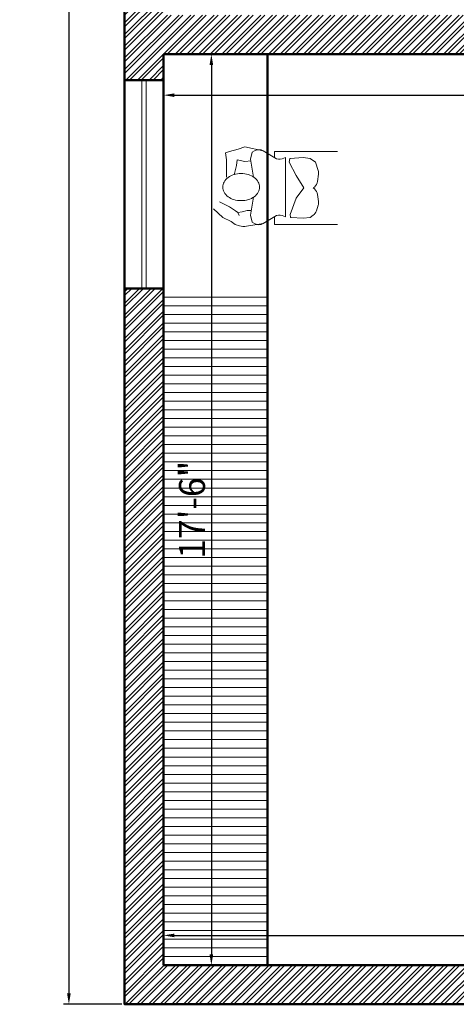
# Model space of a CAD drawing. Units: inches. Extents: x 3590 to 5167, y 65 to 1917.
# Tile 1 of 100: x 3621 to 3722, y 109 to 336. Entities that reach past the tile are written whole.
import ezdxf

# ---------------------------------------------------------------- set-up
doc = ezdxf.new("R2010")
doc.units = ezdxf.units.IN
for name, color, linetype, lineweight in [('A-ANNO-DIMS', 2, 'Continuous', 18), ('A-FURN', 21, 'Continuous', 18), ('A-GLAZ', 4, 'Continuous', 18), ('A-WALL', 7, 'Continuous', 50), ('A-WALL-PATT', 251, 'Continuous', 13)]:
    doc.layers.add(name, color=color, linetype=linetype, lineweight=lineweight)
doc.styles.get("Standard").update_dxf_attribs({"font": 'arial.ttf'})
doc.dimstyles.new('ISO-25', dxfattribs={"dimtxt": 9, "dimasz": 2.5, "dimexe": 1.25, "dimexo": 0.625, "dimtad": 1, "dimdec": 1, "dimlunit": 3, "dimtxsty": 'Standard', "dimcen": 2.5, "dimadec": 0, "dimazin": 0, "dimtfac": 1, "dimtdec": 1, "dimtmove": 0, "dimatfit": 3, "dimfxl": 1, "dimarcsym": 0})

# ---------------------------------------------------------------- blocks, each defined once
blk = doc.blocks.new('*D248')
at = {"layer": 'A-ANNO-DIMS', "color": 0, "lineweight": -2, "transparency": 16777216}
for p, q in [((3644.89, 589.06), (3631.39, 589.06)), ((3632.64, 586.56), (3632.64, 111.56)), ((3644.89, 109.06), (3631.39, 109.06))]:
    blk.add_line(p, q, dxfattribs=at)
at = {"layer": 'A-ANNO-DIMS', "color": 0, "transparency": 16777216}
for points in [[(3632.22, 586.56), (3633.06, 586.56), (3632.64, 589.06)], [(3632.22, 111.56), (3633.06, 111.56), (3632.64, 109.06)]]:
    blk.add_solid(points, dxfattribs=at)
at = {"layer": 'Defpoints', "color": 0, "transparency": 16777216}
for p in [(3645.51, 589.06), (3632.64, 109.06), (3645.51, 109.06)]:
    blk.add_point(p, dxfattribs=at)
at = {"layer": 'A-ANNO-DIMS', "color": 0, "transparency": 16777216, "insert": (3627.42, 349.06), "char_height": 9, "attachment_point": 5, "rotation": 90}
blk.add_mtext("40'", dxfattribs=at)
blk = doc.blocks.new('*D240')
at = {"layer": 'A-ANNO-DIMS', "color": 0, "lineweight": -2, "transparency": 16777216}
for p, q in [((3654.51, 327.43), (3654.51, 317.35)), ((3864.51, 327.43), (3864.51, 317.35)), ((3657.01, 318.6), (3862.01, 318.6))]:
    blk.add_line(p, q, dxfattribs=at)
at = {"layer": 'A-ANNO-DIMS', "color": 0, "transparency": 16777216}
for points in [[(3657.01, 319.02), (3657.01, 318.18), (3654.51, 318.6)], [(3862.01, 319.02), (3862.01, 318.18), (3864.51, 318.6)]]:
    blk.add_solid(points, dxfattribs=at)
at = {"layer": 'Defpoints', "color": 0, "transparency": 16777216}
for p in [(3654.51, 328.06), (3864.51, 328.06), (3864.51, 318.6)]:
    blk.add_point(p, dxfattribs=at)
at = {"layer": 'A-ANNO-DIMS', "color": 0, "transparency": 16777216, "insert": (3759.51, 322.29), "char_height": 6, "attachment_point": 5}
blk.add_mtext('17\'-6"', dxfattribs=at)
blk = doc.blocks.new('*D241')
at = {"layer": 'A-ANNO-DIMS', "color": 0, "lineweight": -2, "transparency": 16777216}
for p, q in [((3655.14, 328.06), (3666.77, 328.06)), ((3665.52, 325.56), (3665.52, 120.56)), ((3655.14, 118.06), (3666.77, 118.06))]:
    blk.add_line(p, q, dxfattribs=at)
at = {"layer": 'A-ANNO-DIMS', "color": 0, "transparency": 16777216}
for points in [[(3665.1, 325.56), (3665.94, 325.56), (3665.52, 328.06)], [(3665.1, 120.56), (3665.94, 120.56), (3665.52, 118.06)]]:
    blk.add_solid(points, dxfattribs=at)
at = {"layer": 'Defpoints', "color": 0, "transparency": 16777216}
for p in [(3654.51, 328.06), (3654.51, 118.06), (3665.52, 118.06)]:
    blk.add_point(p, dxfattribs=at)
at = {"layer": 'A-ANNO-DIMS', "color": 0, "transparency": 16777216, "insert": (3661.83, 223.06), "char_height": 6, "attachment_point": 5, "rotation": 90}
blk.add_mtext('17\'-6"', dxfattribs=at)
blk = doc.blocks.new('*D194')
at = {"layer": 'A-ANNO-DIMS', "color": 0, "lineweight": -2, "transparency": 16777216}
for p, q in [((3654.51, 118.68), (3654.51, 126.19)), ((3657.01, 124.94), (3862.01, 124.94)), ((3864.51, 118.68), (3864.51, 126.19))]:
    blk.add_line(p, q, dxfattribs=at)
at = {"layer": 'A-ANNO-DIMS', "color": 0, "transparency": 16777216}
for points in [[(3657.01, 125.36), (3657.01, 124.52), (3654.51, 124.94)], [(3862.01, 125.36), (3862.01, 124.52), (3864.51, 124.94)]]:
    blk.add_solid(points, dxfattribs=at)
at = {"layer": 'Defpoints', "color": 0, "transparency": 16777216}
for p in [(3864.51, 124.94), (3654.51, 118.06), (3864.51, 118.06)]:
    blk.add_point(p, dxfattribs=at)
at = {"layer": 'A-ANNO-DIMS', "color": 0, "transparency": 16777216, "insert": (3759.51, 128.63), "char_height": 6, "attachment_point": 5}
blk.add_mtext('17\'-6"', dxfattribs=at)

msp = doc.modelspace()

# ---------------------------------------------------------------- hatches: boundary and pattern name
at = {"layer": 'A-WALL-PATT', "transparency": 33554687}
h = msp.add_hatch(dxfattribs=at)
h.set_pattern_fill('ANSI32', color=256, scale=0.2)
h.set_pattern_definition([(45, (0, -1216.9392), (-1.3470384, 1.3470384), []), (45, (0.898, -1216.9392), (-1.3470384, 1.3470384), [])])
h.paths.add_polyline_path([(3768.51, 589.06), (3645.51, 589.06), (3645.51, 568.06), (3654.51, 568.06), (3654.51, 580.06), (3671.16, 580.06), (3768.51, 580.06)])
h.paths.add_polyline_path([(3909.51, 589.06), (3816.51, 589.06), (3816.51, 580.06), (3864.51, 580.06), (3864.51, 574.06), (3873.51, 574.06), (3873.51, 580.06), (3909.51, 580.06)])
h.paths.add_polyline_path([(4053.51, 589.06), (3969.51, 589.06), (3969.51, 580.06), (4053.51, 580.06)])
h.paths.add_polyline_path([(4215.51, 589.06), (4113.51, 589.06), (4113.51, 580.06), (4206.51, 580.06), (4206.51, 574.06), (4215.51, 574.06)])
h.paths.add_polyline_path([(3654.51, 520.06), (3645.51, 520.06), (3645.51, 403.06), (3654.51, 403.06), (3654.51, 433.06), (3741.51, 433.06), (3741.51, 439.06), (3654.51, 439.06)], flags=17)
h.paths.add_polyline_path([(3873.51, 538.06), (3864.51, 538.06), (3864.51, 439.06), (3771.51, 439.06), (3771.51, 433.06), (3774.51, 433.06), (3774.51, 337.06), (3654.51, 337.06), (3654.51, 367.06), (3645.51, 367.06), (3645.51, 322.06), (3654.51, 322.06), (3654.51, 328.06), (3864.51, 328.06), (3864.51, 322.06), (3873.51, 322.06), (3873.51, 367.06), (3864.51, 367.06), (3864.51, 337.06), (3780.51, 337.06), (3780.51, 433.06), (3864.51, 433.06), (3864.51, 403.06), (3873.51, 403.06)])
h.paths.add_polyline_path([(3654.51, 274.06), (3645.51, 274.06), (3645.51, 109.06), (3810.51, 109.06), (3810.51, 118.06), (3809.96, 118.06), (3654.51, 118.06)])
h.paths.add_polyline_path([(3915.51, 118.06), (3873.51, 118.06), (3873.51, 135.93), (3873.51, 205.06), (3876.51, 205.06), (3876.51, 214.06), (3864.51, 214.06), (3864.51, 118.06), (3858.51, 118.06), (3858.51, 109.06), (3915.51, 109.06)])
h.paths.add_polyline_path([(4028.01, 118.06), (4002.51, 118.06), (4002.51, 286.06), (3981.51, 286.06), (3981.51, 277.06), (3993.51, 277.06), (3993.51, 214.06), (3921.51, 214.06), (3921.51, 277.06), (3933.51, 277.06), (3933.51, 286.06), (3864.51, 286.06), (3864.51, 277.06), (3912.51, 277.06), (3912.51, 214.06), (3906.51, 214.06), (3906.51, 205.06), (3993.51, 205.06), (3993.51, 118.06), (3951.51, 118.06), (3951.51, 109.06), (4028.01, 109.06)])
h.paths.add_polyline_path([(4203.51, 118.06), (4158.51, 118.06), (4158.51, 310.06), (4194.51, 310.06), (4194.51, 319.06), (4149.51, 319.06), (4149.51, 118.06), (4124.01, 118.06), (4124.01, 109.06), (4203.51, 109.06)])
h.paths.add_polyline_path([(4305.51, 349.06), (4296.51, 349.06), (4296.51, 319.06), (4278.64, 319.06), (4260.51, 319.06), (4260.51, 310.06), (4296.51, 310.06), (4296.51, 304.06), (4305.51, 304.06)])
h.paths.add_polyline_path([(4305.51, 256.06), (4296.51, 256.06), (4296.51, 118.06), (4251.51, 118.06), (4251.51, 109.06), (4305.51, 109.06)])
h.paths.add_polyline_path([(4305.51, 460.06), (4215.51, 460.06), (4215.51, 526.06), (4206.51, 526.06), (4206.51, 460.06), (4149.51, 460.06), (4149.51, 451.06), (4296.51, 451.06), (4296.51, 421.06), (4305.51, 421.06)])

# ---------------------------------------------------------------- linework, layer by layer
at = {"layer": 'A-FURN'}
for p, q in [((3674.9, 305.46), (3674.54, 303.85)), ((3675.51, 305.8), (3674.9, 305.46)), ((3680.2, 304.14), (3677.49, 305.77)), ((3694.59, 305.64), (3680.09, 305.64)), ((3680.09, 305.64), (3680.09, 304.21)), ((3682.6, 304.21), (3681.85, 303.96)), ((3682.6, 304.21), (3682.6, 290.59)), ((3682.6, 290.59), (3682.6, 304.21)), ((3683.73, 304.03), (3686.72, 304.21)), ((3686.72, 304.21), (3688.33, 304.03)), ((3674.54, 303.85), (3675.25, 299.73)), ((3683.49, 303.13), (3683.66, 303.97)), ((3685.1, 300.09), (3683.49, 303.13)), ((3688.33, 304.03), (3689.58, 303.13)), ((3689.58, 303.13), (3690.17, 301.21)), ((3686.89, 297.22), (3685.1, 300.09)), ((3690.24, 300.38), (3690.04, 298.74)), ((3689.31, 297.43), (3689.04, 297.22)), ((3674.54, 290.95), (3675.25, 295.07)), ((3685.1, 294.89), (3686.89, 297.22)), ((3689.31, 297.01), (3689.04, 297.22)), ((3690.24, 294.06), (3690.04, 295.7)), ((3667.43, 293.99), (3669.7, 292.89)), ((3669.7, 292.89), (3671.06, 291.96)), ((3683.67, 291.13), (3685.1, 294.89)), ((3689.78, 291.95), (3690.17, 293.23)), ((3668.13, 290.43), (3666.04, 292.42)), ((3671.06, 291.96), (3671.66, 291.53)), ((3671.66, 291.53), (3671.96, 290.83)), ((3674.9, 289.34), (3674.54, 290.95)), ((3680.2, 290.66), (3677.49, 289.03)), ((3680.09, 290.59), (3680.09, 288.8)), ((3682.6, 290.59), (3681.85, 290.84)), ((3683.8, 290.46), (3683.67, 291.13)), ((3688.33, 290.41), (3689.03, 290.92)), ((3670.06, 289.46), (3668.13, 290.43)), ((3677.49, 289.03), (3673.14, 288.37)), ((3675.51, 289), (3674.9, 289.34)), ((3680.09, 288.8), (3694.59, 288.8)), ((3683.88, 290.4), (3686.72, 290.23)), ((3686.72, 290.23), (3688.33, 290.41)), ((3678.51, 272.06), (3654.51, 272.06)), ((3678.51, 270.06), (3654.51, 270.06)), ((3678.51, 268.06), (3654.51, 268.06)), ((3678.51, 266.06), (3654.51, 266.06)), ((3678.51, 264.06), (3654.51, 264.06)), ((3678.51, 262.06), (3654.51, 262.06)), ((3678.51, 260.06), (3654.51, 260.06)), ((3678.51, 258.06), (3654.51, 258.06)), ((3678.51, 256.06), (3654.51, 256.06)), ((3678.51, 254.06), (3654.51, 254.06)), ((3678.51, 252.06), (3654.51, 252.06)), ((3678.51, 250.06), (3654.51, 250.06)), ((3678.51, 248.06), (3654.51, 248.06)), ((3678.51, 246.06), (3654.51, 246.06)), ((3678.51, 244.06), (3654.51, 244.06)), ((3678.51, 242.06), (3654.51, 242.06)), ((3678.51, 240.06), (3654.51, 240.06)), ((3678.51, 238.06), (3654.51, 238.06)), ((3678.51, 236.06), (3654.51, 236.06)), ((3678.51, 234.06), (3654.51, 234.06)), ((3678.51, 232.06), (3654.51, 232.06)), ((3678.51, 230.06), (3654.51, 230.06)), ((3678.51, 228.06), (3654.51, 228.06)), ((3678.51, 226.06), (3654.51, 226.06)), ((3678.51, 224.06), (3654.51, 224.06)), ((3678.51, 222.06), (3654.51, 222.06)), ((3678.51, 220.06), (3654.51, 220.06)), ((3678.51, 218.06), (3654.51, 218.06)), ((3678.51, 216.06), (3654.51, 216.06)), ((3678.51, 214.06), (3654.51, 214.06)), ((3678.51, 212.06), (3654.51, 212.06)), ((3678.51, 210.06), (3654.51, 210.06)), ((3678.51, 208.06), (3654.51, 208.06)), ((3678.51, 206.06), (3654.51, 206.06)), ((3678.51, 204.06), (3654.51, 204.06)), ((3678.51, 202.06), (3654.51, 202.06)), ((3678.51, 200.06), (3654.51, 200.06)), ((3678.51, 198.06), (3654.51, 198.06)), ((3678.51, 196.06), (3654.51, 196.06)), ((3678.51, 194.06), (3654.51, 194.06)), ((3678.51, 192.06), (3654.51, 192.06)), ((3678.51, 190.06), (3654.51, 190.06)), ((3678.51, 188.06), (3654.51, 188.06)), ((3678.51, 186.06), (3654.51, 186.06)), ((3678.51, 184.06), (3654.51, 184.06)), ((3678.51, 182.06), (3654.51, 182.06)), ((3678.51, 180.06), (3654.51, 180.06)), ((3678.51, 178.06), (3654.51, 178.06)), ((3678.51, 176.06), (3654.51, 176.06)), ((3678.51, 174.06), (3654.51, 174.06)), ((3678.51, 172.06), (3654.51, 172.06)), ((3678.51, 170.06), (3654.51, 170.06)), ((3678.51, 168.06), (3654.51, 168.06)), ((3678.51, 166.06), (3654.51, 166.06)), ((3678.51, 164.06), (3654.51, 164.06)), ((3678.51, 162.06), (3654.51, 162.06)), ((3678.51, 160.06), (3654.51, 160.06)), ((3678.51, 158.06), (3654.51, 158.06)), ((3678.51, 156.06), (3654.51, 156.06)), ((3678.51, 154.06), (3654.51, 154.06)), ((3678.51, 152.06), (3654.51, 152.06)), ((3678.51, 150.06), (3654.51, 150.06)), ((3678.51, 148.06), (3654.51, 148.06)), ((3678.51, 146.06), (3654.51, 146.06)), ((3678.51, 144.06), (3654.51, 144.06)), ((3678.51, 142.06), (3654.51, 142.06)), ((3678.51, 140.06), (3654.51, 140.06)), ((3678.51, 138.06), (3654.51, 138.06)), ((3678.51, 136.06), (3654.51, 136.06)), ((3678.51, 134.06), (3654.51, 134.06)), ((3678.51, 132.06), (3654.51, 132.06)), ((3678.51, 130.06), (3654.51, 130.06)), ((3678.51, 128.06), (3654.51, 128.06)), ((3678.51, 126.06), (3654.51, 126.06)), ((3678.51, 126.06), (3654.51, 126.06)), ((3678.51, 124.06), (3654.51, 124.06)), ((3678.51, 122.06), (3654.51, 122.06)), ((3678.51, 120.06), (3654.51, 120.06))]:
    msp.add_line(p, q, dxfattribs=at)
for points in [[(3677.49, 305.77), (3673.28, 306.71), (3671.67, 306.18), (3669.7, 305.64), (3668.81, 305.28), (3668.99, 303.67), (3668.99, 302.06), (3668.99, 299.73)], [(3670.78, 300.26), (3671.31, 302.41), (3671.49, 303.67), (3673.28, 303.31), (3674.72, 303.49)], [(3671.66, 291.53), (3672.6, 291.75), (3673.82, 291.99), (3674.7, 291.99)], [(3670.06, 289.46), (3671.04, 288.81), (3672.02, 288.52), (3672.8, 288.37), (3673.24, 288.37)]]:
    msp.add_lwpolyline(points, dxfattribs=at)
msp.add_lwpolyline([(3672.39, 294.29, 0.07405), (3674.07, 294.54, 0.084801), (3675.39, 295.2, 0.106336), (3676.34, 296.27, 0.128955), (3676.64, 297.41, 0.128955), (3676.34, 298.55, 0.106336), (3675.39, 299.62, 0.084801), (3674.07, 300.28, 0.07405), (3672.39, 300.53, 0.07405), (3670.71, 300.28, 0.084801), (3669.39, 299.62, 0.106336), (3668.44, 298.55, 0.128955), (3668.14, 297.41, 0.128955), (3668.44, 296.27, 0.106336), (3669.39, 295.2, 0.084801), (3670.71, 294.54, 0.07405)], format="xyb", close=True, dxfattribs=at)
for centre, radius, start, end in [((3676.47, 304.06), 1.98, 59.0235, 119.0669), ((3681.22, 305.84), 1.98, 239.0235, 288.4436), ((3683.74, 303.95), 0.0779, 93.3682, 168.6956), ((3683.74, 303.95), 0.0779, 93.3682, 168.6956), ((3688.27, 300.63), 1.98, 352.8785, 17.0946), ((3688.07, 298.98), 1.98, 308.6739, 352.8785), ((3688.07, 295.46), 1.98, 7.1215, 51.3261), ((3688.27, 293.81), 1.98, 342.9054, 7.1215), ((3681.22, 288.96), 1.98, 71.5564, 120.9765), ((3687.88, 292.53), 1.98, 305.5514, 342.9054), ((3676.47, 290.73), 1.98, 240.9331, 300.9765), ((3683.88, 290.48), 0.0779, 191.3044, 266.6318)]:
    msp.add_arc(centre, radius, start, end, dxfattribs=at)
at = {"layer": 'A-GLAZ'}
for p, q in [((3649.51, 274.06), (3649.51, 322.06)), ((3650.51, 274.06), (3650.51, 322.06))]:
    msp.add_line(p, q, dxfattribs=at)
at = {"layer": 'A-WALL'}
for p, q in [((3864.51, 328.06), (3654.51, 328.06)), ((3654.51, 118.06), (3654.51, 328.06)), ((3678.51, 118.06), (3678.51, 328.06)), ((3654.51, 322.06), (3645.51, 322.06)), ((3654.51, 274.06), (3645.51, 274.06)), ((3864.51, 118.06), (3654.51, 118.06))]:
    msp.add_line(p, q, dxfattribs=at)
msp.add_lwpolyline([(4305.51, 460.06), (4305.51, 109.06), (3645.51, 109.06), (3645.51, 589.06), (4215.51, 589.06)], dxfattribs=at)

# ---------------------------------------------------------------- dimensions: what is measured, and where the dimension line sits
at = {"layer": 'A-ANNO-DIMS'}
for base, p1, p2, override, picture, middle in [((3632.64, 109.06), (3645.51, 589.06), (3645.51, 109.06), {"dimclrd": 0, "dimclre": 0, "dimclrt": 0}, '*D248', (3627.42, 349.06)), ((3665.52, 118.06), (3654.51, 328.06), (3654.51, 118.06), {"dimtxt": 6, "dimclrd": 0, "dimclre": 0, "dimclrt": 0}, '*D241', (3661.83, 223.06))]:
    dim = msp.add_linear_dim(base=base, p1=p1, p2=p2, angle=90, dimstyle='ISO-25', override=override, dxfattribs=at)
    dim.commit()
    dim.dimension.update_dxf_attribs({"geometry": picture, "text_midpoint": middle})
for base, p1, p2, picture, middle in [((3864.51, 318.6), (3654.51, 328.06), (3864.51, 328.06), '*D240', (3759.51, 322.29)), ((3864.51, 124.94), (3654.51, 118.06), (3864.51, 118.06), '*D194', (3759.51, 128.63))]:
    dim = msp.add_linear_dim(base=base, p1=p1, p2=p2, dimstyle='ISO-25', override={"dimtxt": 6, "dimclrd": 0, "dimclre": 0, "dimclrt": 0}, dxfattribs=at)
    dim.commit()
    dim.dimension.update_dxf_attribs({"geometry": picture, "text_midpoint": middle})

doc.saveas('drawing.dxf')
